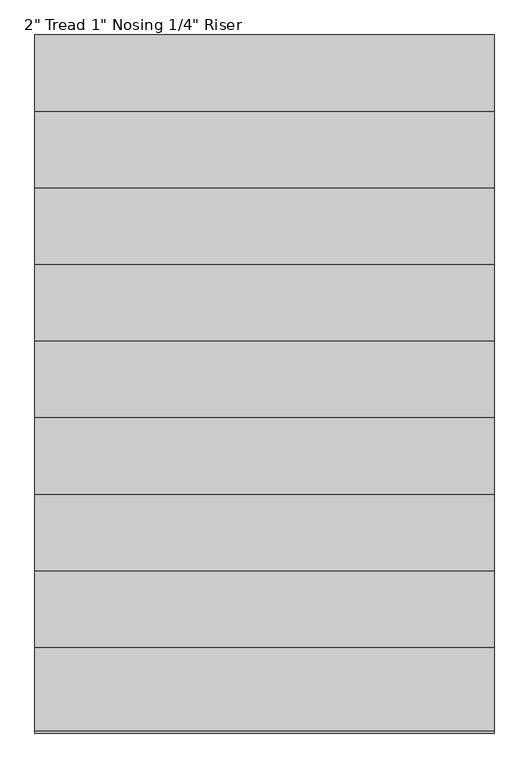
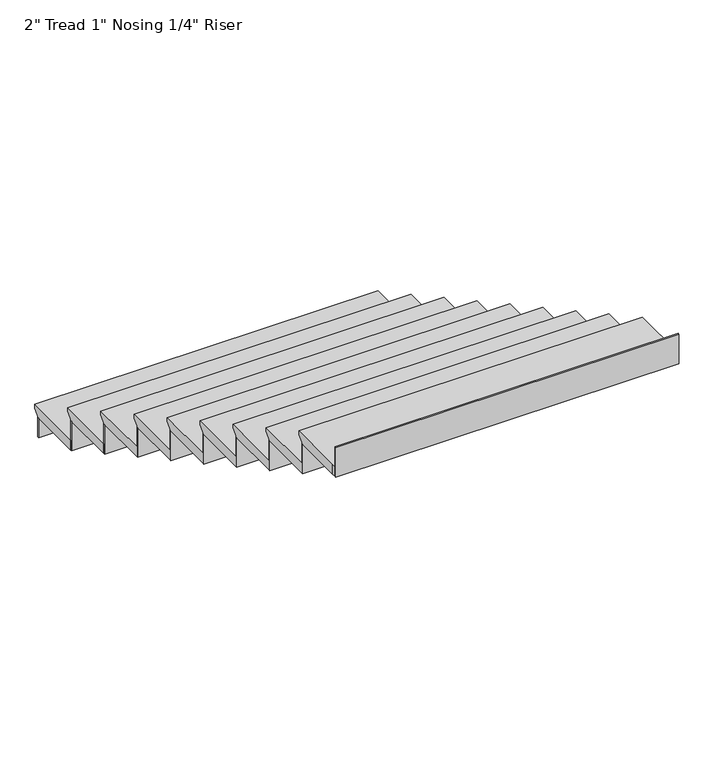
"""IFC4 building model written with IfcOpenShell, lengths in millimetres: stair flight geometry."""

from ifc_helpers import new_model, si_unit, origin, place, context, project, spatial, faceted_brep, source, transform, mapped, element, save


def stair_flight_ae9a2714(model_context):
    return source(origin(), model_context, "Body", "Brep", [
        faceted_brep([(53660.3072437, 33466.7590238, 742.95), (53660.3072437, 33466.7590238, 762.0), (55336.7072437, 33466.7590238, 762.0), (55336.7072437, 33466.7590238, 742.95), (53660.3072437, 33441.3590238, 717.55), (55336.7072437, 33441.3590238, 717.55), (53660.3072437, 33161.9590238, 762.0), (55336.7072437, 33161.9590238, 762.0), (55336.7072437, 33441.3590238, 711.2), (55336.7072437, 33161.9590238, 711.2), (53660.3072437, 33161.9590238, 711.2), (53660.3072437, 33441.3590238, 711.2)], [[[0, 1, 2, 3]], [[4, 0, 3, 5]], [[2, 1, 6, 7]], [[8, 9, 10, 11]], [[2, 7, 9, 8, 5, 3]], [[8, 11, 4, 5]], [[6, 1, 0, 4, 11, 10]], [[7, 6, 10, 9]]]),
        faceted_brep([(53660.3072437, 33441.3590238, 711.2), (53660.3072437, 33441.3590238, 609.6), (53660.3072437, 33435.0090238, 609.6), (53660.3072437, 33435.0090238, 711.2), (55336.7072437, 33441.3590238, 711.2), (55336.7072437, 33435.0090238, 711.2), (55336.7072437, 33435.0090238, 609.6), (55336.7072437, 33441.3590238, 609.6)], [[[0, 1, 2, 3]], [[4, 5, 6, 7]], [[1, 0, 4, 7]], [[2, 1, 7, 6]], [[3, 2, 6, 5]], [[0, 3, 5, 4]]]),
        faceted_brep([(53660.3072437, 33161.9590238, 863.6), (53660.3072437, 33161.9590238, 711.2), (53660.3072437, 33155.6090238, 711.2), (53660.3072437, 33155.6090238, 863.6), (55336.7072437, 33161.9590238, 863.6), (55336.7072437, 33155.6090238, 863.6), (55336.7072437, 33155.6090238, 711.2), (55336.7072437, 33161.9590238, 711.2)], [[[0, 1, 2, 3]], [[4, 5, 6, 7]], [[1, 0, 4, 7]], [[2, 1, 7, 6]], [[3, 2, 6, 5]], [[0, 3, 5, 4]]]),
        faceted_brep([(55336.7072437, 33187.3590238, 914.4), (53660.3072437, 33187.3590238, 914.4), (53660.3072437, 32882.5590238, 914.4), (55336.7072437, 32882.5590238, 914.4), (55336.7072437, 33161.9590238, 863.6), (55336.7072437, 32882.5590238, 863.6), (53660.3072437, 32882.5590238, 863.6), (53660.3072437, 33161.9590238, 863.6), (55336.7072437, 33161.9590238, 869.95), (55336.7072437, 33187.3590238, 895.35), (53660.3072437, 33161.9590238, 869.95), (53660.3072437, 33187.3590238, 895.35)], [[[0, 1, 2, 3]], [[4, 5, 6, 7]], [[0, 3, 5, 4, 8, 9]], [[4, 7, 10, 8]], [[2, 1, 11, 10, 7, 6]], [[3, 2, 6, 5]], [[11, 1, 0, 9]], [[10, 11, 9, 8]]]),
        faceted_brep([(53660.3072437, 32882.5590238, 1016.0), (53660.3072437, 32882.5590238, 863.6), (53660.3072437, 32876.2090238, 863.6), (53660.3072437, 32876.2090238, 1016.0), (55336.7072437, 32882.5590238, 1016.0), (55336.7072437, 32876.2090238, 1016.0), (55336.7072437, 32876.2090238, 863.6), (55336.7072437, 32882.5590238, 863.6)], [[[0, 1, 2, 3]], [[4, 5, 6, 7]], [[1, 0, 4, 7]], [[2, 1, 7, 6]], [[3, 2, 6, 5]], [[0, 3, 5, 4]]]),
        faceted_brep([(55336.7072437, 32907.9590238, 1066.8), (53660.3072437, 32907.9590238, 1066.8), (53660.3072437, 32603.1590238, 1066.8), (55336.7072437, 32603.1590238, 1066.8), (55336.7072437, 32882.5590238, 1016.0), (55336.7072437, 32603.1590238, 1016.0), (53660.3072437, 32603.1590238, 1016.0), (53660.3072437, 32882.5590238, 1016.0), (55336.7072437, 32882.5590238, 1022.35), (55336.7072437, 32907.9590238, 1047.75), (53660.3072437, 32882.5590238, 1022.35), (53660.3072437, 32907.9590238, 1047.75)], [[[0, 1, 2, 3]], [[4, 5, 6, 7]], [[0, 3, 5, 4, 8, 9]], [[4, 7, 10, 8]], [[2, 1, 11, 10, 7, 6]], [[3, 2, 6, 5]], [[11, 1, 0, 9]], [[10, 11, 9, 8]]]),
        faceted_brep([(53660.3072437, 32603.1590238, 1168.4), (53660.3072437, 32603.1590238, 1016.0), (53660.3072437, 32596.8090238, 1016.0), (53660.3072437, 32596.8090238, 1168.4), (55336.7072437, 32603.1590238, 1168.4), (55336.7072437, 32596.8090238, 1168.4), (55336.7072437, 32596.8090238, 1016.0), (55336.7072437, 32603.1590238, 1016.0)], [[[0, 1, 2, 3]], [[4, 5, 6, 7]], [[1, 0, 4, 7]], [[2, 1, 7, 6]], [[3, 2, 6, 5]], [[0, 3, 5, 4]]]),
        faceted_brep([(55336.7072437, 32628.5590238, 1219.2), (53660.3072437, 32628.5590238, 1219.2), (53660.3072437, 32323.7590238, 1219.2), (55336.7072437, 32323.7590238, 1219.2), (55336.7072437, 32603.1590238, 1168.4), (55336.7072437, 32323.7590238, 1168.4), (53660.3072437, 32323.7590238, 1168.4), (53660.3072437, 32603.1590238, 1168.4), (55336.7072437, 32603.1590238, 1174.75), (55336.7072437, 32628.5590238, 1200.15), (53660.3072437, 32603.1590238, 1174.75), (53660.3072437, 32628.5590238, 1200.15)], [[[0, 1, 2, 3]], [[4, 5, 6, 7]], [[0, 3, 5, 4, 8, 9]], [[4, 7, 10, 8]], [[2, 1, 11, 10, 7, 6]], [[3, 2, 6, 5]], [[11, 1, 0, 9]], [[10, 11, 9, 8]]]),
        faceted_brep([(53660.3072437, 32323.7590238, 1320.8), (53660.3072437, 32323.7590238, 1168.4), (53660.3072437, 32317.4090238, 1168.4), (53660.3072437, 32317.4090238, 1320.8), (55336.7072437, 32323.7590238, 1320.8), (55336.7072437, 32317.4090238, 1320.8), (55336.7072437, 32317.4090238, 1168.4), (55336.7072437, 32323.7590238, 1168.4)], [[[0, 1, 2, 3]], [[4, 5, 6, 7]], [[1, 0, 4, 7]], [[2, 1, 7, 6]], [[3, 2, 6, 5]], [[0, 3, 5, 4]]]),
        faceted_brep([(55336.7072437, 32349.1590238, 1371.6), (53660.3072437, 32349.1590238, 1371.6), (53660.3072437, 32044.3590238, 1371.6), (55336.7072437, 32044.3590238, 1371.6), (55336.7072437, 32323.7590238, 1320.8), (55336.7072437, 32044.3590238, 1320.8), (53660.3072437, 32044.3590238, 1320.8), (53660.3072437, 32323.7590238, 1320.8), (55336.7072437, 32323.7590238, 1327.15), (55336.7072437, 32349.1590238, 1352.55), (53660.3072437, 32323.7590238, 1327.15), (53660.3072437, 32349.1590238, 1352.55)], [[[0, 1, 2, 3]], [[4, 5, 6, 7]], [[0, 3, 5, 4, 8, 9]], [[4, 7, 10, 8]], [[2, 1, 11, 10, 7, 6]], [[3, 2, 6, 5]], [[11, 1, 0, 9]], [[10, 11, 9, 8]]]),
        faceted_brep([(53660.3072437, 32044.3590238, 1473.2), (53660.3072437, 32044.3590238, 1320.8), (53660.3072437, 32038.0090238, 1320.8), (53660.3072437, 32038.0090238, 1473.2), (55336.7072437, 32044.3590238, 1473.2), (55336.7072437, 32038.0090238, 1473.2), (55336.7072437, 32038.0090238, 1320.8), (55336.7072437, 32044.3590238, 1320.8)], [[[0, 1, 2, 3]], [[4, 5, 6, 7]], [[1, 0, 4, 7]], [[2, 1, 7, 6]], [[3, 2, 6, 5]], [[0, 3, 5, 4]]]),
        faceted_brep([(55336.7072437, 32069.7590238, 1524.0), (53660.3072437, 32069.7590238, 1524.0), (53660.3072437, 31764.9590238, 1524.0), (55336.7072437, 31764.9590238, 1524.0), (55336.7072437, 32044.3590238, 1473.2), (55336.7072437, 31764.9590238, 1473.2), (53660.3072437, 31764.9590238, 1473.2), (53660.3072437, 32044.3590238, 1473.2), (55336.7072437, 32044.3590238, 1479.55), (55336.7072437, 32069.7590238, 1504.95), (53660.3072437, 32044.3590238, 1479.55), (53660.3072437, 32069.7590238, 1504.95)], [[[0, 1, 2, 3]], [[4, 5, 6, 7]], [[0, 3, 5, 4, 8, 9]], [[4, 7, 10, 8]], [[2, 1, 11, 10, 7, 6]], [[3, 2, 6, 5]], [[11, 1, 0, 9]], [[10, 11, 9, 8]]]),
        faceted_brep([(53660.3072437, 31764.9590238, 1625.6), (53660.3072437, 31764.9590238, 1473.2), (53660.3072437, 31758.6090238, 1473.2), (53660.3072437, 31758.6090238, 1625.6), (55336.7072437, 31764.9590238, 1625.6), (55336.7072437, 31758.6090238, 1625.6), (55336.7072437, 31758.6090238, 1473.2), (55336.7072437, 31764.9590238, 1473.2)], [[[0, 1, 2, 3]], [[4, 5, 6, 7]], [[1, 0, 4, 7]], [[2, 1, 7, 6]], [[3, 2, 6, 5]], [[0, 3, 5, 4]]]),
        faceted_brep([(55336.7072437, 31790.3590238, 1676.4), (53660.3072437, 31790.3590238, 1676.4), (53660.3072437, 31485.5590238, 1676.4), (55336.7072437, 31485.5590238, 1676.4), (55336.7072437, 31764.9590238, 1625.6), (55336.7072437, 31485.5590238, 1625.6), (53660.3072437, 31485.5590238, 1625.6), (53660.3072437, 31764.9590238, 1625.6), (55336.7072437, 31764.9590238, 1631.95), (55336.7072437, 31790.3590238, 1657.35), (53660.3072437, 31764.9590238, 1631.95), (53660.3072437, 31790.3590238, 1657.35)], [[[0, 1, 2, 3]], [[4, 5, 6, 7]], [[0, 3, 5, 4, 8, 9]], [[4, 7, 10, 8]], [[2, 1, 11, 10, 7, 6]], [[3, 2, 6, 5]], [[11, 1, 0, 9]], [[10, 11, 9, 8]]]),
        faceted_brep([(53660.3072437, 31485.5590238, 1778.0), (53660.3072437, 31485.5590238, 1625.6), (53660.3072437, 31479.2090238, 1625.6), (53660.3072437, 31479.2090238, 1778.0), (55336.7072437, 31485.5590238, 1778.0), (55336.7072437, 31479.2090238, 1778.0), (55336.7072437, 31479.2090238, 1625.6), (55336.7072437, 31485.5590238, 1625.6)], [[[0, 1, 2, 3]], [[4, 5, 6, 7]], [[1, 0, 4, 7]], [[2, 1, 7, 6]], [[3, 2, 6, 5]], [[0, 3, 5, 4]]]),
        faceted_brep([(55336.7072437, 31510.9590238, 1828.8), (53660.3072437, 31510.9590238, 1828.8), (53660.3072437, 31206.1590238, 1828.8), (55336.7072437, 31206.1590238, 1828.8), (55336.7072437, 31485.5590238, 1778.0), (55336.7072437, 31206.1590238, 1778.0), (53660.3072437, 31206.1590238, 1778.0), (53660.3072437, 31485.5590238, 1778.0), (55336.7072437, 31485.5590238, 1784.35), (55336.7072437, 31510.9590238, 1809.75), (53660.3072437, 31485.5590238, 1784.35), (53660.3072437, 31510.9590238, 1809.75)], [[[0, 1, 2, 3]], [[4, 5, 6, 7]], [[0, 3, 5, 4, 8, 9]], [[4, 7, 10, 8]], [[2, 1, 11, 10, 7, 6]], [[3, 2, 6, 5]], [[11, 1, 0, 9]], [[10, 11, 9, 8]]]),
        faceted_brep([(53660.3072437, 30926.7590238, 2082.8), (53660.3072437, 30926.7590238, 1930.4), (53660.3072437, 30920.4090238, 1930.4), (53660.3072437, 30920.4090238, 2082.8), (55336.7072437, 30926.7590238, 2082.8), (55336.7072437, 30920.4090238, 2082.8), (55336.7072437, 30920.4090238, 1930.4), (55336.7072437, 30926.7590238, 1930.4)], [[[0, 1, 2, 3]], [[4, 5, 6, 7]], [[1, 0, 4, 7]], [[2, 1, 7, 6]], [[3, 2, 6, 5]], [[0, 3, 5, 4]]]),
        faceted_brep([(53660.3072437, 31206.1590238, 1930.4), (53660.3072437, 31206.1590238, 1778.0), (53660.3072437, 31199.8090238, 1778.0), (53660.3072437, 31199.8090238, 1930.4), (55336.7072437, 31206.1590238, 1930.4), (55336.7072437, 31199.8090238, 1930.4), (55336.7072437, 31199.8090238, 1778.0), (55336.7072437, 31206.1590238, 1778.0)], [[[0, 1, 2, 3]], [[4, 5, 6, 7]], [[1, 0, 4, 7]], [[2, 1, 7, 6]], [[3, 2, 6, 5]], [[0, 3, 5, 4]]]),
        faceted_brep([(55336.7072437, 31231.5590238, 1981.2), (53660.3072437, 31231.5590238, 1981.2), (53660.3072437, 30952.1590238, 1981.2), (53660.3072437, 30926.7590238, 1981.2), (55336.7072437, 30926.7590238, 1981.2), (55336.7072437, 31206.1590238, 1930.4), (55336.7072437, 30926.7590238, 1930.4), (53660.3072437, 30926.7590238, 1930.4), (53660.3072437, 30952.1590238, 1930.4), (53660.3072437, 31206.1590238, 1930.4), (55336.7072437, 31206.1590238, 1936.75), (55336.7072437, 31231.5590238, 1962.15), (53660.3072437, 31206.1590238, 1936.75), (53660.3072437, 31231.5590238, 1962.15)], [[[0, 1, 2, 3, 4]], [[5, 6, 7, 8, 9]], [[0, 4, 6, 5, 10, 11]], [[5, 9, 12, 10]], [[2, 1, 13, 12, 9, 8]], [[3, 2, 8, 7]], [[4, 3, 7, 6]], [[13, 1, 0, 11]], [[12, 13, 11, 10]]]),
    ])


if __name__ == "__main__":
    model = new_model("IFC4")
    model_context = context("Model", 3, world=origin())
    ifc_project = project(units=[si_unit("LENGTHUNIT", "METRE", prefix="MILLI")], contexts=[model_context])
    site = spatial("IfcSite", under=ifc_project)
    building = spatial("IfcBuilding", under=site)
    placement = place(None, origin())
    stair_flight_shape = stair_flight_ae9a2714(model_context)
    element("IfcStairFlight", 1, ObjectType="2\" Tread 1\" Nosing 1/4\" Riser", at=placement, inside=building, context=model_context, shape_type="MappedRepresentation", body=[
        mapped(stair_flight_shape, transform((0.0, 0.0, 0.0), x_axis=(1.0, 0.0, 0.0), y_axis=(0.0, 1.0, 0.0), z_axis=(0.0, 0.0, 1.0))),
    ])
    save(model, "model.ifc")
